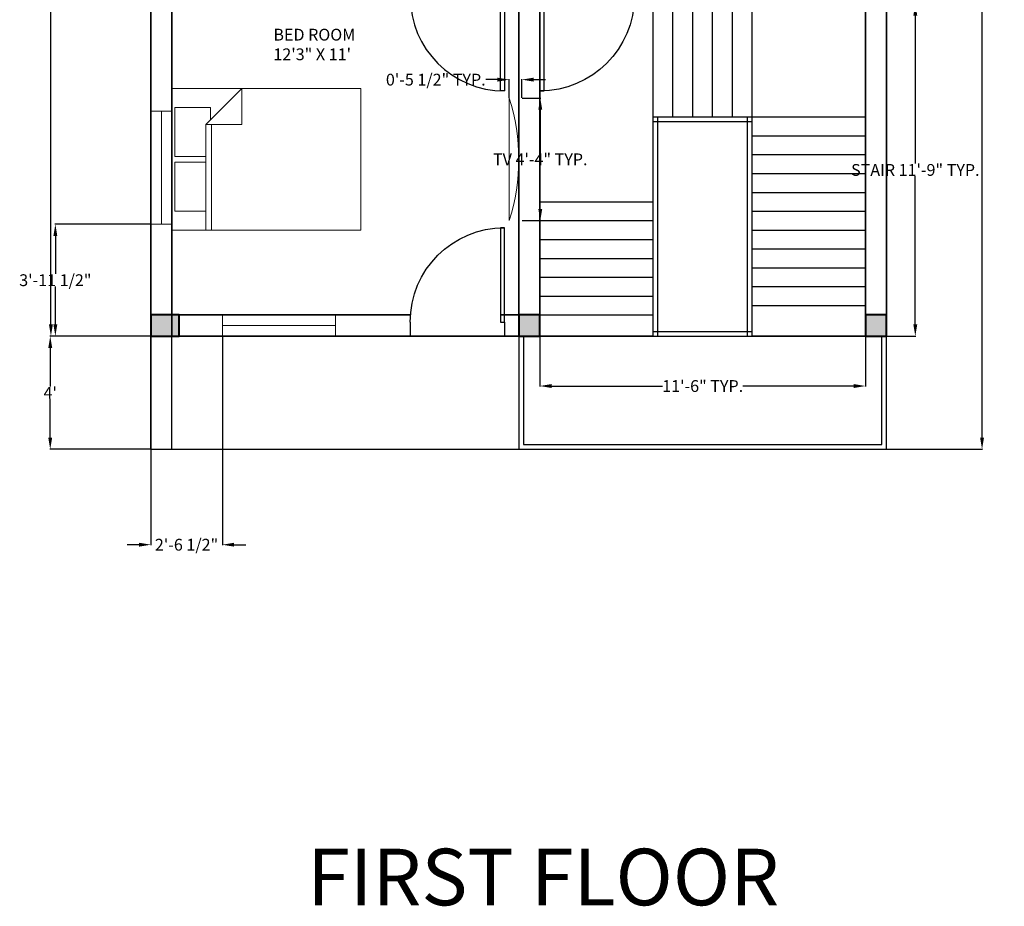
# Model space of a CAD drawing. Units: inches. Extents: x -54 to 881, y -122 to 681.
# Tile 4 of 6: x 464 to 881, y -122 to 254. Entities that reach past the tile are written whole.
import ezdxf

# ---------------------------------------------------------------- set-up
doc = ezdxf.new("R2010")
doc.units = ezdxf.units.IN
doc.header["$MEASUREMENT"] = 0
for name, color, linetype, lineweight in [('A-ANNO-DIMS', 2, 'Continuous', 18), ('A-ANNO-TITL', 7, 'Continuous', 35), ('A-DOOR', 3, 'Continuous', 25), ('A-EQPM', 9, 'Continuous', 18), ('A-FLOR-BALC', 7, 'Continuous', 25), ('A-FLOR-STRS', 7, 'Continuous', 25), ('A-FURN', 8, 'Continuous', 18), ('A-GLAZ', 4, 'Continuous', 20), ('A-WALL', 7, 'Continuous', 35)]:
    doc.layers.add(name, color=color, linetype=linetype, lineweight=lineweight)
doc.layers.add('A-AREA-IDEN', color=217, linetype='Continuous', lineweight=18, true_color=0x93278f)
doc.layers.add('A-COLS', color=240, linetype='Continuous', lineweight=40, true_color=0xed1f24)
doc.styles.get("Standard").update_dxf_attribs({"font": 'arial.ttf'})
doc.dimstyles.get("Standard").update_dxf_attribs({"dimtxt": 5, "dimasz": 5, "dimexe": 0.18, "dimexo": 0.0625, "dimgap": 0.09, "dimtad": 0, "dimtih": 1, "dimtoh": 1, "dimdec": 0, "dimzin": 0, "dimdsep": 46, "dimlunit": 3, "dimtxsty": 'Standard', "dimcen": 0.09, "dimadec": 0, "dimazin": 0, "dimtfac": 1, "dimtdec": 0, "dimtofl": 0, "dimtmove": 0, "dimatfit": 3, "dimfxl": 1, "dimtolj": 1, "dimtzin": 0, "dimarcsym": 0})

# ---------------------------------------------------------------- blocks, each defined once
blk = doc.blocks.new('*D14')
at = {"layer": 'A-ANNO-DIMS', "color": 0, "lineweight": -2, "transparency": 16777216}
for p, q in [((519.43, 624), (476.98, 624)), ((477.16, 619), (477.16, 374.6)), ((477.16, 125), (477.16, 369.4)), ((519.43, 120), (476.98, 120))]:
    blk.add_line(p, q, dxfattribs=at)
at = {"layer": 'A-ANNO-DIMS', "color": 0, "transparency": 16777216}
for points in [[(476.32, 619), (477.99, 619), (477.16, 624)], [(476.32, 125), (477.99, 125), (477.16, 120)]]:
    blk.add_solid(points, dxfattribs=at)
at = {"layer": 'Defpoints', "color": 0, "transparency": 16777216}
for p in [(519.49, 624), (477.16, 120), (519.49, 120)]:
    blk.add_point(p, dxfattribs=at)
at = {"layer": 'A-ANNO-DIMS', "color": 0, "transparency": 16777216, "insert": (477.16, 372), "char_height": 5, "attachment_point": 5}
blk.add_mtext("\\A1;42'", dxfattribs=at)
blk = doc.blocks.new('*U12')
for p, q in [((0, 0), (0, -6)), ((40, 0), (40, -6))]:
    blk.add_line(p, q)
blk.add_lwpolyline([(0, 0), (0, 40), (1.75, 40), (1.75, 0)], close=True)
blk.add_arc((0, 0), 40, 0, 90)
blk = doc.blocks.new('Bed - Queen')
for p, q in [((0, -80.00003), (0, 0)), ((0, 0), (59.99999, 0)), ((59.99999, 0), (59.99999, -80.00003)), ((7.99999, -1.2), (28.79998, -1.2)), ((7.99999, -14.4), (7.99999, -1.2)), ((28.79998, -1.2), (28.79998, -14.4)), ((31.19999, -1.2), (51.99999, -1.2)), ((31.19999, -14.4), (31.19999, -1.2)), ((51.99999, -1.2), (51.99999, -16.4)), ((0, -14.4), (44.8, -14.4)), ((59.99999, -29.6), (44.8, -14.4)), ((44.8, -14.4), (44.8, -29.6)), ((51.99999, -16.4), (46.79936, -16.4)), ((44.8, -16.8), (0, -16.8)), ((44.8, -29.6), (59.99999, -29.6)), ((59.99999, -80.00003), (0, -80.00003))]:
    blk.add_line(p, q)
blk = doc.blocks.new('*D23')
at = {"layer": 'A-ANNO-DIMS', "color": 0, "lineweight": -2, "transparency": 16777216}
for p, q in [((519.43, 120), (476.69, 120)), ((476.87, 115), (476.87, 98.59)), ((476.87, 77), (476.87, 93.41)), ((519.43, 72), (476.69, 72))]:
    blk.add_line(p, q, dxfattribs=at)
at = {"layer": 'A-ANNO-DIMS', "color": 0, "transparency": 16777216}
for points in [[(476.04, 115), (477.71, 115), (476.87, 120)], [(476.04, 77), (477.71, 77), (476.87, 72)]]:
    blk.add_solid(points, dxfattribs=at)
at = {"layer": 'Defpoints', "color": 0, "transparency": 16777216}
for p in [(519.49, 120), (476.87, 72), (519.49, 72)]:
    blk.add_point(p, dxfattribs=at)
at = {"layer": 'A-ANNO-DIMS', "color": 0, "transparency": 16777216, "insert": (476.87, 96), "char_height": 5, "attachment_point": 5}
blk.add_mtext("\\A1;4'", dxfattribs=at)
blk = doc.blocks.new('WIN-48X9')
for p, q in [((0, 0), (0, 9)), ((48, 0), (48, 9)), ((0, 4.5), (48, 4.5))]:
    blk.add_line(p, q)
blk = doc.blocks.new('TV-52-PLAN')
blk.add_line((0, 4), (52, 4))
blk.add_arc((26, 86.41), 86.41, 252.4883, 287.5117)
blk = doc.blocks.new('STAIR-RETURN-FLIGHT')
for p, q in [((48, 93), (48, 141)), ((56.4, 93), (56.4, 141)), ((64.8, 93), (64.8, 141)), ((73.2, 93), (73.2, 141)), ((81.6, 93), (81.6, 141)), ((90, 93), (90, 141)), ((48, 0), (48, 93)), ((48, 93), (90, 93)), ((50, 0), (50, 93)), ((88, 0), (88, 93)), ((90, 0), (90, 93)), ((90, 93), (138, 93)), ((48, 91), (90, 91)), ((90, 85), (138, 85)), ((90, 77), (138, 77)), ((90, 69), (138, 69)), ((90, 61), (138, 61)), ((0, 57), (48, 57)), ((90, 53), (138, 53)), ((0, 49), (48, 49)), ((90, 45), (138, 45)), ((0, 41), (48, 41)), ((90, 37), (138, 37)), ((0, 33), (48, 33)), ((90, 29), (138, 29)), ((0, 25), (48, 25)), ((90, 21), (138, 21)), ((0, 17), (48, 17)), ((90, 13), (138, 13)), ((0, 9), (48, 9)), ((48, 2), (90, 2)), ((48, 0), (90, 0))]:
    blk.add_line(p, q)
blk = doc.blocks.new('COL-9X12')
h = blk.add_hatch(color=256)
h.dxf.hatch_style = 1
h.paths.add_polyline_path([(9, 12), (0, 12), (0, 0), (9, 0)])
blk.add_lwpolyline([(0, 0), (9, 0), (9, 12), (0, 12)], close=True)
blk = doc.blocks.new('COL-9X9')
h = blk.add_hatch(color=256)
h.dxf.hatch_style = 1
h.paths.add_polyline_path([(9, 9), (0, 9), (0, 0), (9, 0)])
blk.add_lwpolyline([(0, 0), (9, 0), (9, 9), (0, 9)], close=True)
blk = doc.blocks.new('*D52')
at = {"layer": 'A-ANNO-DIMS', "color": 0, "lineweight": -2, "transparency": 16777216}
for p, q in [((676.89, 221), (684.81, 221)), ((684.63, 216), (684.63, 197.59)), ((684.63, 174), (684.63, 192.41)), ((676.89, 169), (684.81, 169))]:
    blk.add_line(p, q, dxfattribs=at)
at = {"layer": 'A-ANNO-DIMS', "color": 0, "transparency": 16777216}
for points in [[(683.79, 216), (685.46, 216), (684.63, 221)], [(683.79, 174), (685.46, 174), (684.63, 169)]]:
    blk.add_solid(points, dxfattribs=at)
at = {"layer": 'Defpoints', "color": 0, "transparency": 16777216}
for p in [(676.83, 221), (684.63, 221), (676.83, 169)]:
    blk.add_point(p, dxfattribs=at)
at = {"layer": 'A-ANNO-DIMS', "color": 0, "transparency": 16777216, "insert": (684.63, 195), "char_height": 5, "attachment_point": 5}
blk.add_mtext('\\A1;TV 4\'-4" TYP.', dxfattribs=at)
blk = doc.blocks.new('*D53')
at = {"layer": 'A-ANNO-DIMS', "color": 0, "lineweight": -2, "transparency": 16777216}
for p, q in [((666.49, 228.8), (661.49, 228.8)), ((671.49, 221.06), (671.49, 228.98)), ((676.83, 221.06), (676.83, 228.98)), ((681.83, 228.8), (686.83, 228.8))]:
    blk.add_line(p, q, dxfattribs=at)
at = {"layer": 'A-ANNO-DIMS', "color": 0, "transparency": 16777216}
for points in [[(666.49, 229.63), (666.49, 227.97), (671.49, 228.8)], [(681.83, 229.63), (681.83, 227.97), (676.83, 228.8)]]:
    blk.add_solid(points, dxfattribs=at)
at = {"layer": 'Defpoints', "color": 0, "transparency": 16777216}
for p in [(671.49, 228.8), (671.49, 221), (676.83, 221)]:
    blk.add_point(p, dxfattribs=at)
at = {"layer": 'A-ANNO-DIMS', "color": 0, "transparency": 16777216, "insert": (640.33, 228.8), "char_height": 5, "attachment_point": 5}
blk.add_mtext('\\A1;0\'-5 1/2" TYP.', dxfattribs=at)
blk = doc.blocks.new('*D64')
at = {"layer": 'A-ANNO-DIMS', "color": 0, "lineweight": -2, "transparency": 16777216}
for p, q in [((822.55, 261), (843.82, 261)), ((843.64, 256), (843.64, 193.18)), ((843.64, 125), (843.64, 187.82)), ((822.55, 120), (843.82, 120))]:
    blk.add_line(p, q, dxfattribs=at)
at = {"layer": 'A-ANNO-DIMS', "color": 0, "transparency": 16777216}
for points in [[(842.81, 256), (844.47, 256), (843.64, 261)], [(842.81, 125), (844.47, 125), (843.64, 120)]]:
    blk.add_solid(points, dxfattribs=at)
at = {"layer": 'Defpoints', "color": 0, "transparency": 16777216}
for p in [(822.49, 261), (843.64, 261), (822.49, 120)]:
    blk.add_point(p, dxfattribs=at)
at = {"layer": 'A-ANNO-DIMS', "color": 0, "transparency": 16777216, "insert": (843.64, 190.5), "char_height": 5, "attachment_point": 5}
blk.add_mtext('\\A1;STAIR 11\'-9" TYP.', dxfattribs=at)
blk = doc.blocks.new('*D65')
at = {"layer": 'A-ANNO-DIMS', "color": 0, "lineweight": -2, "transparency": 16777216}
for p, q in [((684.49, 119.94), (684.49, 98.67)), ((822.49, 119.94), (822.49, 98.67)), ((689.49, 98.85), (736.46, 98.85)), ((817.49, 98.85), (770.53, 98.85))]:
    blk.add_line(p, q, dxfattribs=at)
at = {"layer": 'A-ANNO-DIMS', "color": 0, "transparency": 16777216}
for points in [[(689.49, 99.68), (689.49, 98.02), (684.49, 98.85)], [(817.49, 99.68), (817.49, 98.02), (822.49, 98.85)]]:
    blk.add_solid(points, dxfattribs=at)
at = {"layer": 'Defpoints', "color": 0, "transparency": 16777216}
for p in [(684.49, 120), (822.49, 120), (822.49, 98.85)]:
    blk.add_point(p, dxfattribs=at)
at = {"layer": 'A-ANNO-DIMS', "color": 0, "transparency": 16777216, "insert": (753.49, 98.85), "char_height": 5, "attachment_point": 5}
blk.add_mtext('\\A1;11\'-6" TYP.', dxfattribs=at)
blk = doc.blocks.new('*D75')
at = {"layer": 'A-ANNO-DIMS', "color": 0, "lineweight": -2, "transparency": 16777216}
for p, q in [((831.55, 624), (872.12, 624)), ((871.94, 619), (871.94, 350.64)), ((871.94, 77), (871.94, 345.36)), ((831.55, 72), (872.12, 72))]:
    blk.add_line(p, q, dxfattribs=at)
at = {"layer": 'A-ANNO-DIMS', "color": 0, "transparency": 16777216}
for points in [[(871.11, 619), (872.77, 619), (871.94, 624)], [(871.11, 77), (872.77, 77), (871.94, 72)]]:
    blk.add_solid(points, dxfattribs=at)
at = {"layer": 'Defpoints', "color": 0, "transparency": 16777216}
for p in [(831.49, 624), (871.94, 624), (831.49, 72)]:
    blk.add_point(p, dxfattribs=at)
at = {"layer": 'A-ANNO-DIMS', "color": 0, "transparency": 16777216, "insert": (871.94, 348), "char_height": 5, "attachment_point": 5}
blk.add_mtext('\\A1;46\'-0"', dxfattribs=at)
blk = doc.blocks.new('*D87')
at = {"layer": 'A-ANNO-DIMS', "color": 0, "lineweight": -2, "transparency": 16777216}
for p, q in [((519.49, 119.94), (519.49, 31.37)), ((549.84, 119.94), (549.84, 31.37)), ((514.49, 31.55), (509.49, 31.55)), ((554.84, 31.55), (559.84, 31.55))]:
    blk.add_line(p, q, dxfattribs=at)
at = {"layer": 'A-ANNO-DIMS', "color": 0, "transparency": 16777216}
for points in [[(514.49, 32.38), (514.49, 30.72), (519.49, 31.55)], [(554.84, 32.38), (554.84, 30.72), (549.84, 31.55)]]:
    blk.add_solid(points, dxfattribs=at)
at = {"layer": 'Defpoints', "color": 0, "transparency": 16777216}
for p in [(519.49, 120), (549.84, 120), (549.84, 31.55)]:
    blk.add_point(p, dxfattribs=at)
at = {"layer": 'A-ANNO-DIMS', "color": 0, "transparency": 16777216, "insert": (534.66, 31.55), "char_height": 5, "attachment_point": 5}
blk.add_mtext('\\A1;2\'-6 1/2"', dxfattribs=at)
blk = doc.blocks.new('*D88')
at = {"layer": 'A-ANNO-DIMS', "color": 0, "lineweight": -2, "transparency": 16777216}
for p, q in [((519.43, 167.49), (478.86, 167.49)), ((479.04, 162.49), (479.04, 146.42)), ((479.04, 125), (479.04, 141.07)), ((519.43, 120), (478.86, 120))]:
    blk.add_line(p, q, dxfattribs=at)
at = {"layer": 'A-ANNO-DIMS', "color": 0, "transparency": 16777216}
for points in [[(478.21, 162.49), (479.87, 162.49), (479.04, 167.49)], [(478.21, 125), (479.87, 125), (479.04, 120)]]:
    blk.add_solid(points, dxfattribs=at)
at = {"layer": 'Defpoints', "color": 0, "transparency": 16777216}
for p in [(479.04, 167.49), (519.49, 167.49), (519.49, 120)]:
    blk.add_point(p, dxfattribs=at)
at = {"layer": 'A-ANNO-DIMS', "color": 0, "transparency": 16777216, "insert": (479.04, 143.74), "char_height": 5, "attachment_point": 5}
blk.add_mtext('\\A1;3\'-11 1/2"', dxfattribs=at)

msp = doc.modelspace()

# ---------------------------------------------------------------- linework, layer by layer
at = {"layer": 'A-FLOR-BALC'}
for p, q in [((528.49, 72), (528.49, 120)), ((829.49, 74), (829.49, 120)), ((831.49, 72), (831.49, 120))]:
    msp.add_line(p, q, dxfattribs=at)
at = {"layer": 'A-FLOR-BALC', "ltscale": 10}
for p, q in [((675.49, 120), (675.49, 72)), ((677.49, 120), (677.49, 74)), ((519.49, 72), (675.49, 72)), ((675.49, 72), (831.49, 72)), ((677.49, 74), (829.49, 74))]:
    msp.add_line(p, q, dxfattribs=at)
at = {"layer": 'A-WALL'}
for p, q in [((519.49, 72), (519.49, 624)), ((831.49, 120), (831.49, 624)), ((822.49, 120), (822.49, 390)), ((528.49, 120), (528.49, 270)), ((675.49, 120), (675.49, 270)), ((684.49, 120), (684.49, 270)), ((519.49, 129), (629.6, 129)), ((667.74, 129), (684.49, 129)), ((519.49, 120), (732.49, 120)), ((774.49, 120), (831.49, 120))]:
    msp.add_line(p, q, dxfattribs=at)

# ---------------------------------------------------------------- block references
at = {"layer": 'A-COLS', "rotation": 90.00000000000048}
msp.add_blockref('COL-9X12', (531.49, 120), dxfattribs=at)
at = {"layer": 'A-COLS'}
for p in [(675.49, 120), (822.49, 120)]:
    msp.add_blockref('COL-9X9', p, dxfattribs=at)
at = {"layer": 'A-DOOR', "rotation": 180}
msp.add_blockref('*U12', (669.49, 264), dxfattribs=at)
at = {"layer": 'A-DOOR', "xscale": -1, "rotation": 180}
msp.add_blockref('*U12', (684.49, 264), dxfattribs=at)
at = {"layer": 'A-DOOR', "xscale": -1}
msp.add_blockref('*U12', (669.49, 126), dxfattribs=at)
at = {"layer": 'A-EQPM', "rotation": 90}
msp.add_blockref('TV-52-PLAN', (675.49, 169), dxfattribs=at)
at = {"layer": 'A-FLOR-STRS'}
msp.add_blockref('STAIR-RETURN-FLIGHT', (684.49, 120), dxfattribs=at)
at = {"layer": 'A-FURN', "rotation": 90}
msp.add_blockref('Bed - Queen', (528.49, 165), dxfattribs=at)
at = {"layer": 'A-GLAZ'}
for p, rotation in [((528.49, 167.49), 90.00000000000003), ((597.84, 129), 180)]:
    msp.add_blockref('WIN-48X9', p, dxfattribs=dict(at, rotation=rotation))

# ---------------------------------------------------------------- texts
at = {"layer": 'A-ANNO-TITL', "insert": (585.78, -97.4), "char_height": 24, "attachment_point": 1}
msp.add_mtext_dynamic_manual_height_columns('FIRST FLOOR', width=302.3302, gutter_width=1, heights=[0], dxfattribs=at)
at = {"layer": 'A-AREA-IDEN', "insert": (571.49, 250.38), "char_height": 5, "attachment_point": 1}
msp.add_mtext_dynamic_manual_height_columns('BED ROOM\\P12\'3" X 11\'', width=65.2326, gutter_width=1, heights=[0], dxfattribs=at)

# ---------------------------------------------------------------- dimensions: what is measured, and where the dimension line sits
at = {"layer": 'A-ANNO-DIMS'}
for base, p1, p2, override, picture, middle in [((477.16, 120), (519.49, 624), (519.49, 120), {"dimclrd": 0, "dimclre": 0, "dimclrt": 0}, '*D14', (477.16, 372)), ((871.94, 624), (831.49, 72), (831.49, 624), {"dimdec": 1, "dimlfac": 1, "dimrnd": 0, "dimzin": 1, "dimdsep": 46, "dimlunit": 4, "dimfrac": 2}, '*D75', (871.94, 348)), ((479.04, 167.49), (519.49, 120), (519.49, 167.49), {"dimdec": 1, "dimlfac": 1, "dimrnd": 0, "dimzin": 1, "dimdsep": 46, "dimlunit": 4, "dimfrac": 2}, '*D88', (479.04, 143.74)), ((476.87, 72), (519.49, 120), (519.49, 72), {"dimclrd": 0, "dimclre": 0, "dimclrt": 0}, '*D23', (476.87, 96))]:
    dim = msp.add_linear_dim(base=base, p1=p1, p2=p2, angle=90, dimstyle='Standard', override=override, dxfattribs=at)
    dim.commit()
    dim.dimension.update_dxf_attribs({"geometry": picture, "text_midpoint": middle})
for base, p1, p2, angle, text, picture, middle in [((843.64, 261), (822.49, 120), (822.49, 261), 90, 'STAIR <> TYP.', '*D64', (843.64, 190.5)), ((671.49, 228.8), (676.83, 221), (671.49, 221), 180, '<> TYP.', '*D53', (640.33, 228.8)), ((684.63, 221), (676.83, 169), (676.83, 221), 90, 'TV <> TYP.', '*D52', (684.63, 195))]:
    dim = msp.add_linear_dim(base=base, p1=p1, p2=p2, angle=angle, text=text, dimstyle='Standard', override={"dimdec": 1, "dimlfac": 1, "dimrnd": 0, "dimzin": 1, "dimdsep": 46, "dimlunit": 4, "dimfrac": 2}, dxfattribs=at)
    dim.commit()
    dim.dimension.update_dxf_attribs({"geometry": picture, "text_midpoint": middle})
dim = msp.add_linear_dim(base=(549.8384, 31.55), p1=(519.4908, 120), p2=(549.8384, 120), dimstyle='Standard', override={"dimdec": 1, "dimlfac": 1, "dimrnd": 0, "dimzin": 1, "dimdsep": 46, "dimlunit": 4, "dimfrac": 2}, dxfattribs=at)
dim.commit()
dim.dimension.update_dxf_attribs({"geometry": '*D87', "text_midpoint": (534.6646, 31.55)})
dim = msp.add_linear_dim(base=(822.49, 98.85), p1=(684.49, 120), p2=(822.49, 120), text='<> TYP.', dimstyle='Standard', override={"dimdec": 1, "dimlfac": 1, "dimrnd": 0, "dimzin": 1, "dimdsep": 46, "dimlunit": 4, "dimfrac": 2}, dxfattribs=at)
dim.commit()
dim.dimension.update_dxf_attribs({"geometry": '*D65', "text_midpoint": (753.49, 98.85)})

doc.saveas('drawing.dxf')
